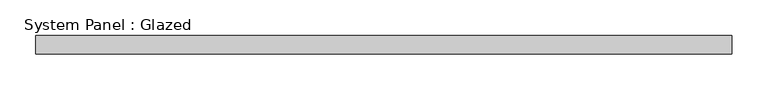
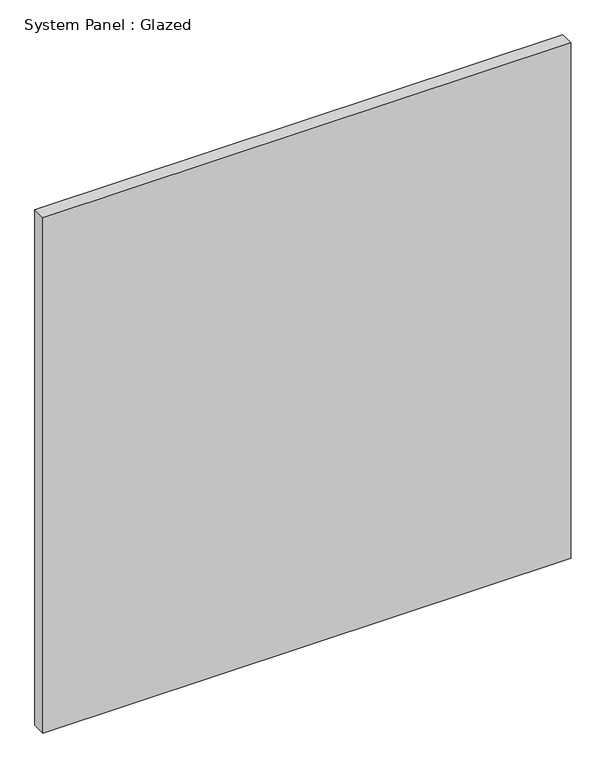
"""IFC4 building model written with IfcOpenShell, lengths in millimetres: plate geometry, System Panel : Glazed."""

from ifc_helpers import new_model, si_unit, origin, origin_with_axes, place, context, project, spatial, polyline, outline, extrude, source, transform, mapped, element, save


def system_panel_glazed_537ed4da(model_context):
    return source(origin(), model_context, "Body", "SweptSolid", [
        extrude(outline(polyline([(485.775, 19.05), (-485.775, 19.05), (-485.775, 44.45), (485.775, 44.45), (485.775, 19.05)])), origin_with_axes(), (0.0, 0.0, 1.0), 1003.3),
    ])


if __name__ == "__main__":
    model = new_model("IFC4")
    model_context = context("Model", 3, world=origin())
    ifc_project = project(units=[si_unit("LENGTHUNIT", "METRE", prefix="MILLI")], contexts=[model_context])
    site = spatial("IfcSite", under=ifc_project)
    building = spatial("IfcBuilding", under=site)
    placement = place(None, origin())
    system_panel_glazed_shape = system_panel_glazed_537ed4da(model_context)
    element("IfcPlate", 1, ObjectType="System Panel : Glazed", at=placement, inside=building, context=model_context, shape_type="MappedRepresentation", body=[
        mapped(system_panel_glazed_shape, transform((0.0, 0.0, 0.0), x_axis=(1.0, 0.0, 0.0), y_axis=(0.0, 1.0, 0.0), z_axis=(0.0, 0.0, 1.0))),
    ])
    save(model, "model.ifc")

# Revit data of these elements
# Type "System Panel : Glazed"
#   Construction Type Id = "GSP4R"
#   Analytic Construction = "1/8 in Pilkington single glazing"
#   Visual Light Transmittance = 0.9
#   Solar Heat Gain Coefficient = 0.86
#   Heat Transfer Coefficient (U) = 1.18115 BTU/(h·ft²·°F)
#   Define Thermal Properties by = 1
# Element 1 (IfcPlate, "System Panel : Glazed")
#   Materials on its faces: "Glass"
# Materials
#   "Glass": class "Glass", colour RGB 0 128 192, transparency 0.75, Description = "Soda Lime Glass", Cost = 0
